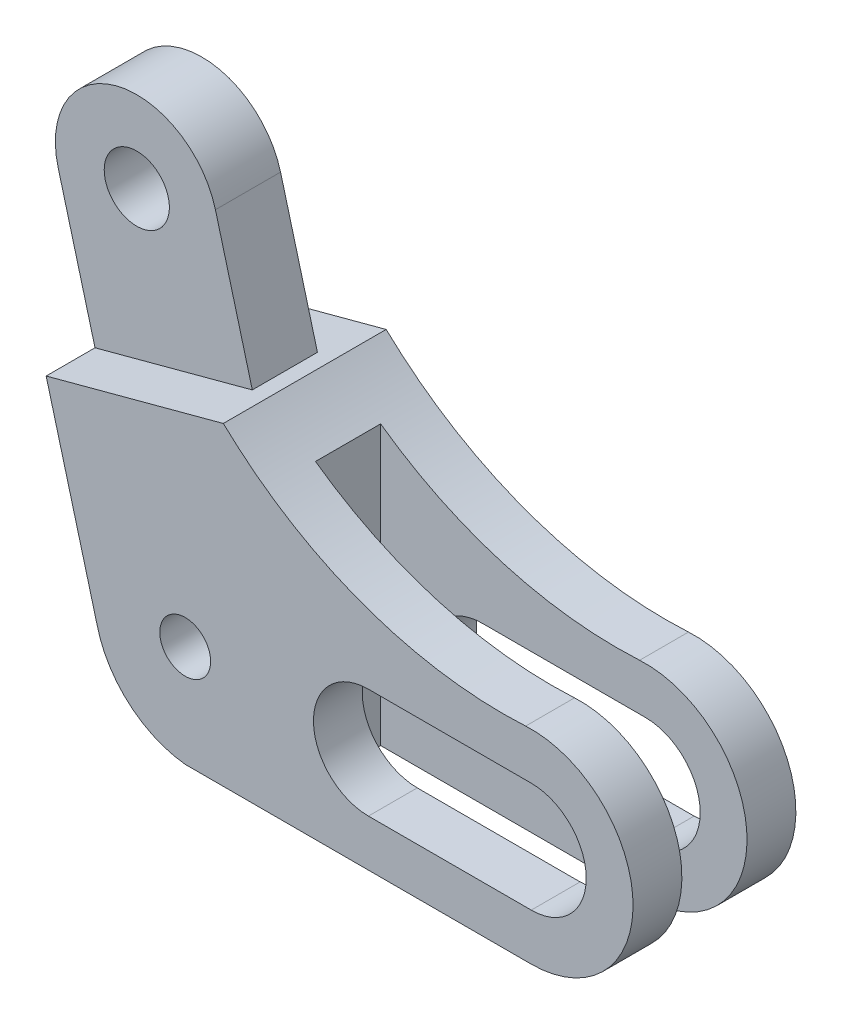
ISO-10303-21;
HEADER;
FILE_DESCRIPTION(('STEP AP214'),'2;1');
FILE_NAME('part.step','',(''),(''),'','','');
FILE_SCHEMA(('AUTOMOTIVE_DESIGN { 1 0 10303 214 1 1 1 1 }'));
ENDSEC;
DATA;
#1=APPLICATION_CONTEXT('core data for automotive mechanical design processes');
#2=APPLICATION_PROTOCOL_DEFINITION('international standard','automotive_design',2000,#1);
#3=PRODUCT_CONTEXT('',#1,'mechanical');
#4=PRODUCT('Part','Part','',(#3));
#5=PRODUCT_RELATED_PRODUCT_CATEGORY('part','',(#4));
#6=PRODUCT_DEFINITION_FORMATION('','',#4);
#7=PRODUCT_DEFINITION_CONTEXT('part definition',#1,'design');
#8=PRODUCT_DEFINITION('design','',#6,#7);
#9=PRODUCT_DEFINITION_SHAPE('','',#8);
#10=(LENGTH_UNIT() NAMED_UNIT(*) SI_UNIT(.MILLI.,.METRE.));
#11=(NAMED_UNIT(*) PLANE_ANGLE_UNIT() SI_UNIT($,.RADIAN.));
#12=(NAMED_UNIT(*) SI_UNIT($,.STERADIAN.) SOLID_ANGLE_UNIT());
#13=UNCERTAINTY_MEASURE_WITH_UNIT(LENGTH_MEASURE(1.E-05),#10,'distance_accuracy_value','');
#14=(GEOMETRIC_REPRESENTATION_CONTEXT(3) GLOBAL_UNCERTAINTY_ASSIGNED_CONTEXT((#13)) GLOBAL_UNIT_ASSIGNED_CONTEXT((#10,
#11,#12)) REPRESENTATION_CONTEXT('',''));
#15=CARTESIAN_POINT('',(0.,0.,0.));
#16=DIRECTION('',(0.,0.,1.));
#17=DIRECTION('',(1.,0.,0.));
#18=AXIS2_PLACEMENT_3D('',#15,#16,#17);
#19=CARTESIAN_POINT('',(0.,0.,20.));
#20=DIRECTION('',(0.,0.,-1.));
#21=DIRECTION('',(-1.,0.,0.));
#22=AXIS2_PLACEMENT_3D('',#19,#20,#21);
#23=CYLINDRICAL_SURFACE('',#22,25.);
#24=CARTESIAN_POINT('',(0.,0.,-8.));
#25=DIRECTION('',(0.,0.,1.));
#26=DIRECTION('',(1.,0.,0.));
#27=AXIS2_PLACEMENT_3D('',#24,#25,#26);
#28=CIRCLE('',#27,25.);
#29=CARTESIAN_POINT('',(0.,-25.,-8.));
#30=VERTEX_POINT('',#29);
#31=CARTESIAN_POINT('',(-1.37615473662768,24.9620952273814,-8.));
#32=VERTEX_POINT('',#31);
#33=EDGE_CURVE('E232',#30,#32,#28,.T.);
#34=ORIENTED_EDGE('',*,*,#33,.F.);
#35=DIRECTION('',(0.,0.,-1.));
#36=VECTOR('',#35,1.);
#37=CARTESIAN_POINT('',(0.,-25.,20.));
#38=LINE('',#37,#36);
#39=CARTESIAN_POINT('',(0.,-25.,-20.));
#40=VERTEX_POINT('',#39);
#41=EDGE_CURVE('E330',#30,#40,#38,.T.);
#42=ORIENTED_EDGE('',*,*,#41,.T.);
#43=CARTESIAN_POINT('',(0.,0.,-20.));
#44=DIRECTION('',(0.,0.,1.));
#45=DIRECTION('',(1.,0.,0.));
#46=AXIS2_PLACEMENT_3D('',#43,#44,#45);
#47=CIRCLE('',#46,25.);
#48=CARTESIAN_POINT('',(-1.37615473662768,24.9620952273814,-20.));
#49=VERTEX_POINT('',#48);
#50=EDGE_CURVE('E309',#40,#49,#47,.T.);
#51=ORIENTED_EDGE('',*,*,#50,.T.);
#52=DIRECTION('',(0.,0.,-1.));
#53=VECTOR('',#52,1.);
#54=CARTESIAN_POINT('',(-1.37615473662768,24.9620952273814,20.));
#55=LINE('',#54,#53);
#56=EDGE_CURVE('E355',#32,#49,#55,.T.);
#57=ORIENTED_EDGE('',*,*,#56,.F.);
#58=EDGE_LOOP('',(#34,#42,#51,#57));
#59=FACE_BOUND('',#58,.T.);
#60=ADVANCED_FACE('F39',(#59),#23,.T.);
#61=CARTESIAN_POINT('',(-6.88077368313851,124.810476136907,20.));
#62=DIRECTION('',(0.,0.,-1.));
#63=DIRECTION('',(-1.,0.,0.));
#64=AXIS2_PLACEMENT_3D('',#61,#62,#63);
#65=CYLINDRICAL_SURFACE('',#64,100.);
#66=CARTESIAN_POINT('',(-6.88077368313851,124.810476136907,-8.));
#67=DIRECTION('',(0.,0.,-1.));
#68=DIRECTION('',(1.,0.,0.));
#69=AXIS2_PLACEMENT_3D('',#66,#67,#68);
#70=CIRCLE('',#69,100.);
#71=CARTESIAN_POINT('',(-65.,43.433848458381,-8.));
#72=VERTEX_POINT('',#71);
#73=EDGE_CURVE('E223',#32,#72,#70,.T.);
#74=ORIENTED_EDGE('',*,*,#73,.F.);
#75=ORIENTED_EDGE('',*,*,#56,.T.);
#76=CARTESIAN_POINT('',(-6.88077368313851,124.810476136907,-20.));
#77=DIRECTION('',(0.,0.,-1.));
#78=DIRECTION('',(-1.,0.,0.));
#79=AXIS2_PLACEMENT_3D('',#76,#77,#78);
#80=CIRCLE('',#79,100.);
#81=CARTESIAN_POINT('',(-75.6404006582522,52.2011537447842,-20.));
#82=VERTEX_POINT('',#81);
#83=EDGE_CURVE('E329',#49,#82,#80,.T.);
#84=ORIENTED_EDGE('',*,*,#83,.T.);
#85=DIRECTION('',(0.,0.,-1.));
#86=VECTOR('',#85,1.);
#87=CARTESIAN_POINT('',(-75.6404006582522,52.2011537447842,20.));
#88=LINE('',#87,#86);
#89=CARTESIAN_POINT('',(-75.6404006582522,52.2011537447842,20.));
#90=VERTEX_POINT('',#89);
#91=EDGE_CURVE('E353',#90,#82,#88,.T.);
#92=ORIENTED_EDGE('',*,*,#91,.F.);
#93=CARTESIAN_POINT('',(-6.88077368313851,124.810476136907,20.));
#94=DIRECTION('',(0.,0.,-1.));
#95=DIRECTION('',(-1.,0.,0.));
#96=AXIS2_PLACEMENT_3D('',#93,#94,#95);
#97=CIRCLE('',#96,100.);
#98=CARTESIAN_POINT('',(-1.37615473662768,24.9620952273814,20.));
#99=VERTEX_POINT('',#98);
#100=EDGE_CURVE('E316',#99,#90,#97,.T.);
#101=ORIENTED_EDGE('',*,*,#100,.F.);
#102=CARTESIAN_POINT('',(-1.37615473662768,24.9620952273814,8.));
#103=VERTEX_POINT('',#102);
#104=EDGE_CURVE('E351',#99,#103,#55,.T.);
#105=ORIENTED_EDGE('',*,*,#104,.T.);
#106=CARTESIAN_POINT('',(-6.88077368313851,124.810476136907,8.));
#107=DIRECTION('',(0.,0.,-1.));
#108=DIRECTION('',(1.,0.,0.));
#109=AXIS2_PLACEMENT_3D('',#106,#107,#108);
#110=CIRCLE('',#109,100.);
#111=CARTESIAN_POINT('',(-65.,43.433848458381,8.));
#112=VERTEX_POINT('',#111);
#113=EDGE_CURVE('E193',#103,#112,#110,.T.);
#114=ORIENTED_EDGE('',*,*,#113,.T.);
#115=DIRECTION('',(0.,0.,1.));
#116=VECTOR('',#115,1.);
#117=CARTESIAN_POINT('',(-65.,43.433848458381,-8.));
#118=LINE('',#117,#116);
#119=EDGE_CURVE('E237',#72,#112,#118,.T.);
#120=ORIENTED_EDGE('',*,*,#119,.F.);
#121=EDGE_LOOP('',(#74,#75,#84,#92,#101,#105,#114,#120));
#122=FACE_BOUND('',#121,.T.);
#123=ADVANCED_FACE('F396',(#122),#65,.F.);
#124=CARTESIAN_POINT('',(0.,-25.,20.));
#125=DIRECTION('',(0.,1.,0.));
#126=DIRECTION('',(-1.,0.,0.));
#127=AXIS2_PLACEMENT_3D('',#124,#125,#126);
#128=PLANE('',#127);
#129=DIRECTION('',(1.,0.,0.));
#130=VECTOR('',#129,1.);
#131=CARTESIAN_POINT('',(-65.,-25.,-8.));
#132=LINE('',#131,#130);
#133=CARTESIAN_POINT('',(-65.,-25.,-8.));
#134=VERTEX_POINT('',#133);
#135=EDGE_CURVE('E235',#134,#30,#132,.T.);
#136=ORIENTED_EDGE('',*,*,#135,.F.);
#137=DIRECTION('',(0.,0.,1.));
#138=VECTOR('',#137,1.);
#139=CARTESIAN_POINT('',(-65.,-25.,-8.));
#140=LINE('',#139,#138);
#141=CARTESIAN_POINT('',(-65.,-25.,8.));
#142=VERTEX_POINT('',#141);
#143=EDGE_CURVE('E250',#134,#142,#140,.T.);
#144=ORIENTED_EDGE('',*,*,#143,.T.);
#145=DIRECTION('',(1.,0.,0.));
#146=VECTOR('',#145,1.);
#147=CARTESIAN_POINT('',(-65.,-25.,8.));
#148=LINE('',#147,#146);
#149=CARTESIAN_POINT('',(0.,-25.,8.));
#150=VERTEX_POINT('',#149);
#151=EDGE_CURVE('E244',#142,#150,#148,.T.);
#152=ORIENTED_EDGE('',*,*,#151,.T.);
#153=CARTESIAN_POINT('',(0.,-25.,20.));
#154=VERTEX_POINT('',#153);
#155=EDGE_CURVE('E336',#154,#150,#38,.T.);
#156=ORIENTED_EDGE('',*,*,#155,.F.);
#157=DIRECTION('',(1.,0.,0.));
#158=VECTOR('',#157,1.);
#159=CARTESIAN_POINT('',(0.,-25.,20.));
#160=LINE('',#159,#158);
#161=CARTESIAN_POINT('',(-85.,-25.,20.));
#162=VERTEX_POINT('',#161);
#163=EDGE_CURVE('E324',#162,#154,#160,.T.);
#164=ORIENTED_EDGE('',*,*,#163,.F.);
#165=DIRECTION('',(0.,0.,-1.));
#166=VECTOR('',#165,1.);
#167=CARTESIAN_POINT('',(-85.,-25.,20.));
#168=LINE('',#167,#166);
#169=CARTESIAN_POINT('',(-85.,-25.,-20.));
#170=VERTEX_POINT('',#169);
#171=EDGE_CURVE('E343',#162,#170,#168,.T.);
#172=ORIENTED_EDGE('',*,*,#171,.T.);
#173=DIRECTION('',(1.,0.,0.));
#174=VECTOR('',#173,1.);
#175=CARTESIAN_POINT('',(0.,-25.,-20.));
#176=LINE('',#175,#174);
#177=EDGE_CURVE('E320',#170,#40,#176,.T.);
#178=ORIENTED_EDGE('',*,*,#177,.T.);
#179=ORIENTED_EDGE('',*,*,#41,.F.);
#180=EDGE_LOOP('',(#136,#144,#152,#156,#164,#172,#178,#179));
#181=FACE_BOUND('',#180,.T.);
#182=ADVANCED_FACE('F405',(#181),#128,.F.);
#183=CARTESIAN_POINT('',(-40.,0.,-20.));
#184=DIRECTION('',(0.,0.,1.));
#185=DIRECTION('',(1.,0.,0.));
#186=AXIS2_PLACEMENT_3D('',#183,#184,#185);
#187=CYLINDRICAL_SURFACE('',#186,13.5);
#188=CARTESIAN_POINT('',(-40.,0.,-8.));
#189=DIRECTION('',(0.,0.,1.));
#190=DIRECTION('',(1.,0.,0.));
#191=AXIS2_PLACEMENT_3D('',#188,#189,#190);
#192=CIRCLE('',#191,13.5);
#193=CARTESIAN_POINT('',(-40.,-13.5,-8.));
#194=VERTEX_POINT('',#193);
#195=CARTESIAN_POINT('',(-40.,13.5,-8.));
#196=VERTEX_POINT('',#195);
#197=EDGE_CURVE('E262',#194,#196,#192,.F.);
#198=ORIENTED_EDGE('',*,*,#197,.F.);
#199=DIRECTION('',(0.,0.,1.));
#200=VECTOR('',#199,1.);
#201=CARTESIAN_POINT('',(-40.,-13.5,-20.));
#202=LINE('',#201,#200);
#203=CARTESIAN_POINT('',(-40.,-13.5,-20.));
#204=VERTEX_POINT('',#203);
#205=EDGE_CURVE('E302',#204,#194,#202,.T.);
#206=ORIENTED_EDGE('',*,*,#205,.F.);
#207=CARTESIAN_POINT('',(-40.,0.,-20.));
#208=DIRECTION('',(0.,0.,1.));
#209=DIRECTION('',(1.,0.,0.));
#210=AXIS2_PLACEMENT_3D('',#207,#208,#209);
#211=CIRCLE('',#210,13.5);
#212=CARTESIAN_POINT('',(-40.,13.5,-20.));
#213=VERTEX_POINT('',#212);
#214=EDGE_CURVE('E270',#213,#204,#211,.T.);
#215=ORIENTED_EDGE('',*,*,#214,.F.);
#216=DIRECTION('',(0.,0.,1.));
#217=VECTOR('',#216,1.);
#218=CARTESIAN_POINT('',(-40.,13.5,-20.));
#219=LINE('',#218,#217);
#220=EDGE_CURVE('E292',#213,#196,#219,.T.);
#221=ORIENTED_EDGE('',*,*,#220,.T.);
#222=EDGE_LOOP('',(#198,#206,#215,#221));
#223=FACE_BOUND('',#222,.T.);
#224=ADVANCED_FACE('F393',(#223),#187,.F.);
#225=CARTESIAN_POINT('',(-40.,13.5,-20.));
#226=DIRECTION('',(0.,1.,0.));
#227=DIRECTION('',(0.,0.,1.));
#228=AXIS2_PLACEMENT_3D('',#225,#226,#227);
#229=PLANE('',#228);
#230=DIRECTION('',(1.,0.,0.));
#231=VECTOR('',#230,1.);
#232=CARTESIAN_POINT('',(-40.,13.5,-8.));
#233=LINE('',#232,#231);
#234=CARTESIAN_POINT('',(0.,13.5,-8.));
#235=VERTEX_POINT('',#234);
#236=EDGE_CURVE('E265',#196,#235,#233,.T.);
#237=ORIENTED_EDGE('',*,*,#236,.F.);
#238=ORIENTED_EDGE('',*,*,#220,.F.);
#239=DIRECTION('',(-1.,0.,0.));
#240=VECTOR('',#239,1.);
#241=CARTESIAN_POINT('',(-40.,13.5,-20.));
#242=LINE('',#241,#240);
#243=CARTESIAN_POINT('',(0.,13.5,-20.));
#244=VERTEX_POINT('',#243);
#245=EDGE_CURVE('E280',#244,#213,#242,.T.);
#246=ORIENTED_EDGE('',*,*,#245,.F.);
#247=DIRECTION('',(0.,0.,1.));
#248=VECTOR('',#247,1.);
#249=CARTESIAN_POINT('',(0.,13.5,-20.));
#250=LINE('',#249,#248);
#251=EDGE_CURVE('E298',#244,#235,#250,.T.);
#252=ORIENTED_EDGE('',*,*,#251,.T.);
#253=EDGE_LOOP('',(#237,#238,#246,#252));
#254=FACE_BOUND('',#253,.T.);
#255=ADVANCED_FACE('F385',(#254),#229,.F.);
#256=CARTESIAN_POINT('',(0.,0.,-20.));
#257=DIRECTION('',(0.,0.,1.));
#258=DIRECTION('',(1.,0.,0.));
#259=AXIS2_PLACEMENT_3D('',#256,#257,#258);
#260=CYLINDRICAL_SURFACE('',#259,13.5);
#261=CARTESIAN_POINT('',(0.,0.,-8.));
#262=DIRECTION('',(0.,0.,1.));
#263=DIRECTION('',(1.,0.,0.));
#264=AXIS2_PLACEMENT_3D('',#261,#262,#263);
#265=CIRCLE('',#264,13.5);
#266=CARTESIAN_POINT('',(0.,-13.5,-8.));
#267=VERTEX_POINT('',#266);
#268=EDGE_CURVE('E257',#235,#267,#265,.F.);
#269=ORIENTED_EDGE('',*,*,#268,.F.);
#270=ORIENTED_EDGE('',*,*,#251,.F.);
#271=CARTESIAN_POINT('',(0.,0.,-20.));
#272=DIRECTION('',(0.,0.,1.));
#273=DIRECTION('',(1.,0.,0.));
#274=AXIS2_PLACEMENT_3D('',#271,#272,#273);
#275=CIRCLE('',#274,13.5);
#276=CARTESIAN_POINT('',(0.,-13.5,-20.));
#277=VERTEX_POINT('',#276);
#278=EDGE_CURVE('E273',#277,#244,#275,.T.);
#279=ORIENTED_EDGE('',*,*,#278,.F.);
#280=DIRECTION('',(0.,0.,1.));
#281=VECTOR('',#280,1.);
#282=CARTESIAN_POINT('',(0.,-13.5,-20.));
#283=LINE('',#282,#281);
#284=EDGE_CURVE('E296',#277,#267,#283,.T.);
#285=ORIENTED_EDGE('',*,*,#284,.T.);
#286=EDGE_LOOP('',(#269,#270,#279,#285));
#287=FACE_BOUND('',#286,.T.);
#288=ADVANCED_FACE('F389',(#287),#260,.F.);
#289=CARTESIAN_POINT('',(-40.,-13.5,-20.));
#290=DIRECTION('',(0.,-1.,0.));
#291=DIRECTION('',(0.,0.,-1.));
#292=AXIS2_PLACEMENT_3D('',#289,#290,#291);
#293=PLANE('',#292);
#294=DIRECTION('',(-1.,0.,0.));
#295=VECTOR('',#294,1.);
#296=CARTESIAN_POINT('',(-40.,-13.5,-8.));
#297=LINE('',#296,#295);
#298=EDGE_CURVE('E11',#267,#194,#297,.T.);
#299=ORIENTED_EDGE('',*,*,#298,.F.);
#300=ORIENTED_EDGE('',*,*,#284,.F.);
#301=DIRECTION('',(1.,0.,0.));
#302=VECTOR('',#301,1.);
#303=CARTESIAN_POINT('',(-40.,-13.5,-20.));
#304=LINE('',#303,#302);
#305=EDGE_CURVE('E269',#204,#277,#304,.T.);
#306=ORIENTED_EDGE('',*,*,#305,.F.);
#307=ORIENTED_EDGE('',*,*,#205,.T.);
#308=EDGE_LOOP('',(#299,#300,#306,#307));
#309=FACE_BOUND('',#308,.T.);
#310=ADVANCED_FACE('F462',(#309),#293,.F.);
#311=CARTESIAN_POINT('',(0.,0.,20.));
#312=DIRECTION('',(0.,0.,1.));
#313=DIRECTION('',(1.,0.,0.));
#314=AXIS2_PLACEMENT_3D('',#311,#312,#313);
#315=PLANE('',#314);
#316=CARTESIAN_POINT('',(-40.,0.,20.));
#317=DIRECTION('',(0.,0.,1.));
#318=DIRECTION('',(1.,0.,0.));
#319=AXIS2_PLACEMENT_3D('',#316,#317,#318);
#320=CIRCLE('',#319,13.5);
#321=CARTESIAN_POINT('',(-40.,13.5,20.));
#322=VERTEX_POINT('',#321);
#323=CARTESIAN_POINT('',(-40.,-13.5,20.));
#324=VERTEX_POINT('',#323);
#325=EDGE_CURVE('E266',#322,#324,#320,.T.);
#326=ORIENTED_EDGE('',*,*,#325,.F.);
#327=DIRECTION('',(-1.,0.,0.));
#328=VECTOR('',#327,1.);
#329=CARTESIAN_POINT('',(-40.,13.5,20.));
#330=LINE('',#329,#328);
#331=CARTESIAN_POINT('',(0.,13.5,20.));
#332=VERTEX_POINT('',#331);
#333=EDGE_CURVE('E271',#332,#322,#330,.T.);
#334=ORIENTED_EDGE('',*,*,#333,.F.);
#335=CARTESIAN_POINT('',(0.,0.,20.));
#336=DIRECTION('',(0.,0.,1.));
#337=DIRECTION('',(1.,0.,0.));
#338=AXIS2_PLACEMENT_3D('',#335,#336,#337);
#339=CIRCLE('',#338,13.5);
#340=CARTESIAN_POINT('',(0.,-13.5,20.));
#341=VERTEX_POINT('',#340);
#342=EDGE_CURVE('E286',#341,#332,#339,.T.);
#343=ORIENTED_EDGE('',*,*,#342,.F.);
#344=DIRECTION('',(1.,0.,0.));
#345=VECTOR('',#344,1.);
#346=CARTESIAN_POINT('',(-40.,-13.5,20.));
#347=LINE('',#346,#345);
#348=EDGE_CURVE('E282',#324,#341,#347,.T.);
#349=ORIENTED_EDGE('',*,*,#348,.F.);
#350=EDGE_LOOP('',(#326,#334,#343,#349));
#351=FACE_BOUND('',#350,.T.);
#352=CARTESIAN_POINT('',(0.,0.,20.));
#353=DIRECTION('',(0.,0.,1.));
#354=DIRECTION('',(1.,0.,0.));
#355=AXIS2_PLACEMENT_3D('',#352,#353,#354);
#356=CIRCLE('',#355,25.);
#357=EDGE_CURVE('E311',#154,#99,#356,.T.);
#358=ORIENTED_EDGE('',*,*,#357,.T.);
#359=ORIENTED_EDGE('',*,*,#100,.T.);
#360=DIRECTION('',(-0.965925826289068,-0.258819045102521,0.));
#361=VECTOR('',#360,1.);
#362=CARTESIAN_POINT('',(-119.156645256425,40.5410111470685,20.));
#363=LINE('',#362,#361);
#364=CARTESIAN_POINT('',(-119.156645256425,40.5410111470685,20.));
#365=VERTEX_POINT('',#364);
#366=EDGE_CURVE('E317',#90,#365,#363,.T.);
#367=ORIENTED_EDGE('',*,*,#366,.T.);
#368=DIRECTION('',(0.258819045102522,-0.965925826289068,0.));
#369=VECTOR('',#368,1.);
#370=CARTESIAN_POINT('',(-106.733331091504,-5.82342851480675,20.));
#371=LINE('',#370,#369);
#372=CARTESIAN_POINT('',(-106.733331091504,-5.82342851480675,20.));
#373=VERTEX_POINT('',#372);
#374=EDGE_CURVE('E321',#365,#373,#371,.T.);
#375=ORIENTED_EDGE('',*,*,#374,.T.);
#376=CARTESIAN_POINT('',(-82.3886864264471,-0.136753200344534,20.));
#377=DIRECTION('',(0.,0.,1.));
#378=DIRECTION('',(-1.,0.,0.));
#379=AXIS2_PLACEMENT_3D('',#376,#377,#378);
#380=CIRCLE('',#379,25.);
#381=EDGE_CURVE('E323',#373,#162,#380,.T.);
#382=ORIENTED_EDGE('',*,*,#381,.T.);
#383=ORIENTED_EDGE('',*,*,#163,.T.);
#384=EDGE_LOOP('',(#358,#359,#367,#375,#382,#383));
#385=FACE_BOUND('',#384,.T.);
#386=CARTESIAN_POINT('',(-85.,0.,20.));
#387=DIRECTION('',(0.,0.,1.));
#388=DIRECTION('',(1.,0.,0.));
#389=AXIS2_PLACEMENT_3D('',#386,#387,#388);
#390=CIRCLE('',#389,6.25);
#391=CARTESIAN_POINT('',(-78.75,0.,20.));
#392=VERTEX_POINT('',#391);
#393=EDGE_CURVE('E307',#392,#392,#390,.T.);
#394=ORIENTED_EDGE('',*,*,#393,.F.);
#395=EDGE_LOOP('',(#394));
#396=FACE_BOUND('',#395,.T.);
#397=ADVANCED_FACE('F375',(#351,#385,#396),#315,.T.);
#398=CARTESIAN_POINT('',(0.,0.,-20.));
#399=DIRECTION('',(0.,0.,1.));
#400=DIRECTION('',(1.,0.,0.));
#401=AXIS2_PLACEMENT_3D('',#398,#399,#400);
#402=PLANE('',#401);
#403=ORIENTED_EDGE('',*,*,#245,.T.);
#404=ORIENTED_EDGE('',*,*,#214,.T.);
#405=ORIENTED_EDGE('',*,*,#305,.T.);
#406=ORIENTED_EDGE('',*,*,#278,.T.);
#407=EDGE_LOOP('',(#403,#404,#405,#406));
#408=FACE_BOUND('',#407,.T.);
#409=ORIENTED_EDGE('',*,*,#50,.F.);
#410=ORIENTED_EDGE('',*,*,#177,.F.);
#411=CARTESIAN_POINT('',(-82.3886864264471,-0.136753200344534,-20.));
#412=DIRECTION('',(0.,0.,1.));
#413=DIRECTION('',(-1.,0.,0.));
#414=AXIS2_PLACEMENT_3D('',#411,#412,#413);
#415=CIRCLE('',#414,25.);
#416=CARTESIAN_POINT('',(-106.733331091504,-5.82342851480675,-20.));
#417=VERTEX_POINT('',#416);
#418=EDGE_CURVE('E338',#417,#170,#415,.T.);
#419=ORIENTED_EDGE('',*,*,#418,.F.);
#420=DIRECTION('',(0.258819045102522,-0.965925826289068,0.));
#421=VECTOR('',#420,1.);
#422=CARTESIAN_POINT('',(-106.733331091504,-5.82342851480675,-20.));
#423=LINE('',#422,#421);
#424=CARTESIAN_POINT('',(-119.156645256425,40.5410111470685,-20.));
#425=VERTEX_POINT('',#424);
#426=EDGE_CURVE('E331',#425,#417,#423,.T.);
#427=ORIENTED_EDGE('',*,*,#426,.F.);
#428=DIRECTION('',(-0.965925826289068,-0.258819045102521,0.));
#429=VECTOR('',#428,1.);
#430=CARTESIAN_POINT('',(-119.156645256425,40.5410111470685,-20.));
#431=LINE('',#430,#429);
#432=EDGE_CURVE('E335',#82,#425,#431,.T.);
#433=ORIENTED_EDGE('',*,*,#432,.F.);
#434=ORIENTED_EDGE('',*,*,#83,.F.);
#435=EDGE_LOOP('',(#409,#410,#419,#427,#433,#434));
#436=FACE_BOUND('',#435,.T.);
#437=CARTESIAN_POINT('',(-85.,0.,-20.));
#438=DIRECTION('',(0.,0.,1.));
#439=DIRECTION('',(1.,0.,0.));
#440=AXIS2_PLACEMENT_3D('',#437,#438,#439);
#441=CIRCLE('',#440,6.25);
#442=CARTESIAN_POINT('',(-78.75,0.,-20.));
#443=VERTEX_POINT('',#442);
#444=EDGE_CURVE('E294',#443,#443,#441,.T.);
#445=ORIENTED_EDGE('',*,*,#444,.T.);
#446=EDGE_LOOP('',(#445));
#447=FACE_BOUND('',#446,.T.);
#448=ADVANCED_FACE('F408',(#408,#436,#447),#402,.F.);
#449=ORIENTED_EDGE('',*,*,#155,.T.);
#450=CARTESIAN_POINT('',(0.,0.,8.));
#451=DIRECTION('',(0.,0.,1.));
#452=DIRECTION('',(1.,0.,0.));
#453=AXIS2_PLACEMENT_3D('',#450,#451,#452);
#454=CIRCLE('',#453,25.);
#455=EDGE_CURVE('E230',#150,#103,#454,.T.);
#456=ORIENTED_EDGE('',*,*,#455,.T.);
#457=ORIENTED_EDGE('',*,*,#104,.F.);
#458=ORIENTED_EDGE('',*,*,#357,.F.);
#459=EDGE_LOOP('',(#449,#456,#457,#458));
#460=FACE_BOUND('',#459,.T.);
#461=ADVANCED_FACE('F41',(#460),#23,.T.);
#462=CARTESIAN_POINT('',(-119.156645256425,40.5410111470685,20.));
#463=DIRECTION('',(0.258819045102521,-0.965925826289068,0.));
#464=DIRECTION('',(0.965925826289068,0.258819045102521,0.));
#465=AXIS2_PLACEMENT_3D('',#462,#463,#464);
#466=PLANE('',#465);
#467=DIRECTION('',(0.,0.,-1.));
#468=VECTOR('',#467,1.);
#469=CARTESIAN_POINT('',(-119.156645256425,40.5410111470685,20.));
#470=LINE('',#469,#468);
#471=CARTESIAN_POINT('',(-119.156645256425,40.5410111470685,-8.));
#472=VERTEX_POINT('',#471);
#473=EDGE_CURVE('E58',#472,#425,#470,.T.);
#474=ORIENTED_EDGE('',*,*,#473,.F.);
#475=DIRECTION('',(0.965925826289068,0.258819045102521,0.));
#476=VECTOR('',#475,1.);
#477=CARTESIAN_POINT('',(-80.5196122048624,50.8937729511694,-8.));
#478=LINE('',#477,#476);
#479=CARTESIAN_POINT('',(-80.5196122048624,50.8937729511694,-8.));
#480=VERTEX_POINT('',#479);
#481=EDGE_CURVE('E54',#472,#480,#478,.T.);
#482=ORIENTED_EDGE('',*,*,#481,.T.);
#483=DIRECTION('',(0.,0.,-1.));
#484=VECTOR('',#483,1.);
#485=CARTESIAN_POINT('',(-80.5196122048624,50.8937729511694,8.));
#486=LINE('',#485,#484);
#487=CARTESIAN_POINT('',(-80.5196122048624,50.8937729511694,8.));
#488=VERTEX_POINT('',#487);
#489=EDGE_CURVE('E183',#488,#480,#486,.T.);
#490=ORIENTED_EDGE('',*,*,#489,.F.);
#491=DIRECTION('',(0.965925826289068,0.258819045102521,0.));
#492=VECTOR('',#491,1.);
#493=CARTESIAN_POINT('',(-80.5196122048624,50.8937729511694,8.));
#494=LINE('',#493,#492);
#495=CARTESIAN_POINT('',(-119.156645256425,40.5410111470685,8.));
#496=VERTEX_POINT('',#495);
#497=EDGE_CURVE('E186',#496,#488,#494,.T.);
#498=ORIENTED_EDGE('',*,*,#497,.F.);
#499=EDGE_CURVE('E349',#365,#496,#470,.T.);
#500=ORIENTED_EDGE('',*,*,#499,.F.);
#501=ORIENTED_EDGE('',*,*,#366,.F.);
#502=ORIENTED_EDGE('',*,*,#91,.T.);
#503=ORIENTED_EDGE('',*,*,#432,.T.);
#504=EDGE_LOOP('',(#474,#482,#490,#498,#500,#501,#502,#503));
#505=FACE_BOUND('',#504,.T.);
#506=ADVANCED_FACE('F189',(#505),#466,.F.);
#507=CARTESIAN_POINT('',(-106.733331091504,-5.82342851480675,20.));
#508=DIRECTION('',(0.965925826289068,0.258819045102522,0.));
#509=DIRECTION('',(-0.258819045102522,0.965925826289068,0.));
#510=AXIS2_PLACEMENT_3D('',#507,#508,#509);
#511=PLANE('',#510);
#512=ORIENTED_EDGE('',*,*,#426,.T.);
#513=DIRECTION('',(0.,0.,-1.));
#514=VECTOR('',#513,1.);
#515=CARTESIAN_POINT('',(-106.733331091504,-5.82342851480675,20.));
#516=LINE('',#515,#514);
#517=EDGE_CURVE('E347',#373,#417,#516,.T.);
#518=ORIENTED_EDGE('',*,*,#517,.F.);
#519=ORIENTED_EDGE('',*,*,#374,.F.);
#520=ORIENTED_EDGE('',*,*,#499,.T.);
#521=DIRECTION('',(0.258819045102522,-0.965925826289068,0.));
#522=VECTOR('',#521,1.);
#523=CARTESIAN_POINT('',(-119.156645256425,40.5410111470685,8.));
#524=LINE('',#523,#522);
#525=CARTESIAN_POINT('',(-128.215311835013,74.348415067186,8.));
#526=VERTEX_POINT('',#525);
#527=EDGE_CURVE('E210',#526,#496,#524,.T.);
#528=ORIENTED_EDGE('',*,*,#527,.F.);
#529=DIRECTION('',(0.,0.,-1.));
#530=VECTOR('',#529,1.);
#531=CARTESIAN_POINT('',(-128.215311835013,74.348415067186,8.));
#532=LINE('',#531,#530);
#533=CARTESIAN_POINT('',(-128.215311835013,74.348415067186,-8.));
#534=VERTEX_POINT('',#533);
#535=EDGE_CURVE('E220',#526,#534,#532,.T.);
#536=ORIENTED_EDGE('',*,*,#535,.T.);
#537=DIRECTION('',(0.258819045102522,-0.965925826289068,0.));
#538=VECTOR('',#537,1.);
#539=CARTESIAN_POINT('',(-119.156645256425,40.5410111470685,-8.));
#540=LINE('',#539,#538);
#541=EDGE_CURVE('E208',#534,#472,#540,.T.);
#542=ORIENTED_EDGE('',*,*,#541,.T.);
#543=ORIENTED_EDGE('',*,*,#473,.T.);
#544=EDGE_LOOP('',(#512,#518,#519,#520,#528,#536,#542,#543));
#545=FACE_BOUND('',#544,.T.);
#546=ADVANCED_FACE('F415',(#545),#511,.F.);
#547=CARTESIAN_POINT('',(-82.3886864264471,-0.136753200344534,20.));
#548=DIRECTION('',(0.,0.,-1.));
#549=DIRECTION('',(-1.,0.,0.));
#550=AXIS2_PLACEMENT_3D('',#547,#548,#549);
#551=CYLINDRICAL_SURFACE('',#550,25.);
#552=ORIENTED_EDGE('',*,*,#418,.T.);
#553=ORIENTED_EDGE('',*,*,#171,.F.);
#554=ORIENTED_EDGE('',*,*,#381,.F.);
#555=ORIENTED_EDGE('',*,*,#517,.T.);
#556=EDGE_LOOP('',(#552,#553,#554,#555));
#557=FACE_BOUND('',#556,.T.);
#558=ADVANCED_FACE('F440',(#557),#551,.T.);
#559=CARTESIAN_POINT('',(-85.,0.,20.));
#560=DIRECTION('',(0.,0.,-1.));
#561=DIRECTION('',(-1.,0.,0.));
#562=AXIS2_PLACEMENT_3D('',#559,#560,#561);
#563=CYLINDRICAL_SURFACE('',#562,6.25);
#564=ORIENTED_EDGE('',*,*,#393,.T.);
#565=EDGE_LOOP('',(#564));
#566=FACE_BOUND('',#565,.T.);
#567=ORIENTED_EDGE('',*,*,#444,.F.);
#568=EDGE_LOOP('',(#567));
#569=FACE_BOUND('',#568,.T.);
#570=ADVANCED_FACE('F386',(#566,#569),#563,.F.);
#571=CARTESIAN_POINT('',(-40.,-13.5,8.));
#572=VERTEX_POINT('',#571);
#573=EDGE_CURVE('E278',#572,#324,#202,.T.);
#574=ORIENTED_EDGE('',*,*,#573,.F.);
#575=CARTESIAN_POINT('',(-40.,0.,8.));
#576=DIRECTION('',(0.,0.,1.));
#577=DIRECTION('',(1.,0.,0.));
#578=AXIS2_PLACEMENT_3D('',#575,#576,#577);
#579=CIRCLE('',#578,13.5);
#580=CARTESIAN_POINT('',(-40.,13.5,8.));
#581=VERTEX_POINT('',#580);
#582=EDGE_CURVE('E260',#572,#581,#579,.F.);
#583=ORIENTED_EDGE('',*,*,#582,.T.);
#584=EDGE_CURVE('E293',#581,#322,#219,.T.);
#585=ORIENTED_EDGE('',*,*,#584,.T.);
#586=ORIENTED_EDGE('',*,*,#325,.T.);
#587=EDGE_LOOP('',(#574,#583,#585,#586));
#588=FACE_BOUND('',#587,.T.);
#589=ADVANCED_FACE('F364',(#588),#187,.F.);
#590=ORIENTED_EDGE('',*,*,#584,.F.);
#591=DIRECTION('',(1.,0.,0.));
#592=VECTOR('',#591,1.);
#593=CARTESIAN_POINT('',(-40.,13.5,8.));
#594=LINE('',#593,#592);
#595=CARTESIAN_POINT('',(0.,13.5,8.));
#596=VERTEX_POINT('',#595);
#597=EDGE_CURVE('E255',#581,#596,#594,.T.);
#598=ORIENTED_EDGE('',*,*,#597,.T.);
#599=EDGE_CURVE('E300',#596,#332,#250,.T.);
#600=ORIENTED_EDGE('',*,*,#599,.T.);
#601=ORIENTED_EDGE('',*,*,#333,.T.);
#602=EDGE_LOOP('',(#590,#598,#600,#601));
#603=FACE_BOUND('',#602,.T.);
#604=ADVANCED_FACE('F377',(#603),#229,.F.);
#605=ORIENTED_EDGE('',*,*,#599,.F.);
#606=CARTESIAN_POINT('',(0.,0.,8.));
#607=DIRECTION('',(0.,0.,1.));
#608=DIRECTION('',(1.,0.,0.));
#609=AXIS2_PLACEMENT_3D('',#606,#607,#608);
#610=CIRCLE('',#609,13.5);
#611=CARTESIAN_POINT('',(0.,-13.5,8.));
#612=VERTEX_POINT('',#611);
#613=EDGE_CURVE('E249',#596,#612,#610,.F.);
#614=ORIENTED_EDGE('',*,*,#613,.T.);
#615=EDGE_CURVE('E303',#612,#341,#283,.T.);
#616=ORIENTED_EDGE('',*,*,#615,.T.);
#617=ORIENTED_EDGE('',*,*,#342,.T.);
#618=EDGE_LOOP('',(#605,#614,#616,#617));
#619=FACE_BOUND('',#618,.T.);
#620=ADVANCED_FACE('F376',(#619),#260,.F.);
#621=ORIENTED_EDGE('',*,*,#615,.F.);
#622=DIRECTION('',(-1.,0.,0.));
#623=VECTOR('',#622,1.);
#624=CARTESIAN_POINT('',(-40.,-13.5,8.));
#625=LINE('',#624,#623);
#626=EDGE_CURVE('E48',#612,#572,#625,.T.);
#627=ORIENTED_EDGE('',*,*,#626,.T.);
#628=ORIENTED_EDGE('',*,*,#573,.T.);
#629=ORIENTED_EDGE('',*,*,#348,.T.);
#630=EDGE_LOOP('',(#621,#627,#628,#629));
#631=FACE_BOUND('',#630,.T.);
#632=ADVANCED_FACE('F362',(#631),#293,.F.);
#633=CARTESIAN_POINT('',(-6.88077368313851,124.810476136907,-8.));
#634=DIRECTION('',(0.,0.,1.));
#635=DIRECTION('',(1.,0.,0.));
#636=AXIS2_PLACEMENT_3D('',#633,#634,#635);
#637=PLANE('',#636);
#638=ORIENTED_EDGE('',*,*,#73,.T.);
#639=DIRECTION('',(0.,-1.,0.));
#640=VECTOR('',#639,1.);
#641=CARTESIAN_POINT('',(-65.,43.433848458381,-8.));
#642=LINE('',#641,#640);
#643=EDGE_CURVE('E227',#72,#134,#642,.T.);
#644=ORIENTED_EDGE('',*,*,#643,.T.);
#645=ORIENTED_EDGE('',*,*,#135,.T.);
#646=ORIENTED_EDGE('',*,*,#33,.T.);
#647=EDGE_LOOP('',(#638,#644,#645,#646));
#648=FACE_BOUND('',#647,.T.);
#649=ORIENTED_EDGE('',*,*,#197,.T.);
#650=ORIENTED_EDGE('',*,*,#236,.T.);
#651=ORIENTED_EDGE('',*,*,#268,.T.);
#652=ORIENTED_EDGE('',*,*,#298,.T.);
#653=EDGE_LOOP('',(#649,#650,#651,#652));
#654=FACE_BOUND('',#653,.T.);
#655=ADVANCED_FACE('F447',(#648,#654),#637,.T.);
#656=CARTESIAN_POINT('',(-6.88077368313851,124.810476136907,8.));
#657=DIRECTION('',(0.,0.,1.));
#658=DIRECTION('',(1.,0.,0.));
#659=AXIS2_PLACEMENT_3D('',#656,#657,#658);
#660=PLANE('',#659);
#661=ORIENTED_EDGE('',*,*,#113,.F.);
#662=ORIENTED_EDGE('',*,*,#455,.F.);
#663=ORIENTED_EDGE('',*,*,#151,.F.);
#664=DIRECTION('',(0.,-1.,0.));
#665=VECTOR('',#664,1.);
#666=CARTESIAN_POINT('',(-65.,43.433848458381,8.));
#667=LINE('',#666,#665);
#668=EDGE_CURVE('E239',#112,#142,#667,.T.);
#669=ORIENTED_EDGE('',*,*,#668,.F.);
#670=EDGE_LOOP('',(#661,#662,#663,#669));
#671=FACE_BOUND('',#670,.T.);
#672=ORIENTED_EDGE('',*,*,#626,.F.);
#673=ORIENTED_EDGE('',*,*,#613,.F.);
#674=ORIENTED_EDGE('',*,*,#597,.F.);
#675=ORIENTED_EDGE('',*,*,#582,.F.);
#676=EDGE_LOOP('',(#672,#673,#674,#675));
#677=FACE_BOUND('',#676,.T.);
#678=ADVANCED_FACE('F380',(#671,#677),#660,.F.);
#679=CARTESIAN_POINT('',(-65.,43.433848458381,-8.));
#680=DIRECTION('',(-1.,0.,0.));
#681=DIRECTION('',(0.,-1.,0.));
#682=AXIS2_PLACEMENT_3D('',#679,#680,#681);
#683=PLANE('',#682);
#684=ORIENTED_EDGE('',*,*,#668,.T.);
#685=ORIENTED_EDGE('',*,*,#143,.F.);
#686=ORIENTED_EDGE('',*,*,#643,.F.);
#687=ORIENTED_EDGE('',*,*,#119,.T.);
#688=EDGE_LOOP('',(#684,#685,#686,#687));
#689=FACE_BOUND('',#688,.T.);
#690=ADVANCED_FACE('F422',(#689),#683,.F.);
#691=CARTESIAN_POINT('',(-89.5782787834506,84.7011768712868,8.));
#692=DIRECTION('',(-0.965925826289068,-0.258819045102522,0.));
#693=DIRECTION('',(0.258819045102522,-0.965925826289068,0.));
#694=AXIS2_PLACEMENT_3D('',#691,#692,#693);
#695=PLANE('',#694);
#696=DIRECTION('',(-0.258819045102521,0.965925826289068,0.));
#697=VECTOR('',#696,1.);
#698=CARTESIAN_POINT('',(-89.5782787834506,84.7011768712868,-8.));
#699=LINE('',#698,#697);
#700=CARTESIAN_POINT('',(-89.5782787834506,84.7011768712868,-8.));
#701=VERTEX_POINT('',#700);
#702=EDGE_CURVE('E218',#480,#701,#699,.T.);
#703=ORIENTED_EDGE('',*,*,#702,.T.);
#704=DIRECTION('',(0.,0.,-1.));
#705=VECTOR('',#704,1.);
#706=CARTESIAN_POINT('',(-89.5782787834506,84.7011768712868,8.));
#707=LINE('',#706,#705);
#708=CARTESIAN_POINT('',(-89.5782787834506,84.7011768712868,8.));
#709=VERTEX_POINT('',#708);
#710=EDGE_CURVE('E192',#709,#701,#707,.T.);
#711=ORIENTED_EDGE('',*,*,#710,.F.);
#712=DIRECTION('',(-0.258819045102521,0.965925826289068,0.));
#713=VECTOR('',#712,1.);
#714=CARTESIAN_POINT('',(-89.5782787834506,84.7011768712868,8.));
#715=LINE('',#714,#713);
#716=EDGE_CURVE('E197',#488,#709,#715,.T.);
#717=ORIENTED_EDGE('',*,*,#716,.F.);
#718=ORIENTED_EDGE('',*,*,#489,.T.);
#719=EDGE_LOOP('',(#703,#711,#717,#718));
#720=FACE_BOUND('',#719,.T.);
#721=ADVANCED_FACE('F196',(#720),#695,.F.);
#722=CARTESIAN_POINT('',(-108.896795309232,79.5247959692363,8.));
#723=DIRECTION('',(0.,0.,-1.));
#724=DIRECTION('',(-1.,0.,0.));
#725=AXIS2_PLACEMENT_3D('',#722,#723,#724);
#726=CYLINDRICAL_SURFACE('',#725,20.);
#727=CARTESIAN_POINT('',(-108.896795309232,79.5247959692363,-8.));
#728=DIRECTION('',(0.,0.,1.));
#729=DIRECTION('',(-1.,0.,0.));
#730=AXIS2_PLACEMENT_3D('',#727,#728,#729);
#731=CIRCLE('',#730,20.);
#732=EDGE_CURVE('E209',#701,#534,#731,.T.);
#733=ORIENTED_EDGE('',*,*,#732,.T.);
#734=ORIENTED_EDGE('',*,*,#535,.F.);
#735=CARTESIAN_POINT('',(-108.896795309232,79.5247959692363,8.));
#736=DIRECTION('',(0.,0.,1.));
#737=DIRECTION('',(-1.,0.,0.));
#738=AXIS2_PLACEMENT_3D('',#735,#736,#737);
#739=CIRCLE('',#738,20.);
#740=EDGE_CURVE('E205',#709,#526,#739,.T.);
#741=ORIENTED_EDGE('',*,*,#740,.F.);
#742=ORIENTED_EDGE('',*,*,#710,.T.);
#743=EDGE_LOOP('',(#733,#734,#741,#742));
#744=FACE_BOUND('',#743,.T.);
#745=ADVANCED_FACE('F511',(#744),#726,.T.);
#746=CARTESIAN_POINT('',(-108.896795309232,79.5247959692363,8.));
#747=DIRECTION('',(0.,0.,-1.));
#748=DIRECTION('',(-1.,0.,0.));
#749=AXIS2_PLACEMENT_3D('',#746,#747,#748);
#750=PLANE('',#749);
#751=CARTESIAN_POINT('',(-108.896795309232,79.5247959692363,8.00000000000001));
#752=DIRECTION('',(0.,0.,-1.));
#753=DIRECTION('',(-1.,0.,0.));
#754=AXIS2_PLACEMENT_3D('',#751,#752,#753);
#755=CIRCLE('',#754,8.);
#756=CARTESIAN_POINT('',(-116.896795309232,79.5247959692363,8.00000000000001));
#757=VERTEX_POINT('',#756);
#758=EDGE_CURVE('E213',#757,#757,#755,.T.);
#759=ORIENTED_EDGE('',*,*,#758,.T.);
#760=EDGE_LOOP('',(#759));
#761=FACE_BOUND('',#760,.T.);
#762=ORIENTED_EDGE('',*,*,#497,.T.);
#763=ORIENTED_EDGE('',*,*,#716,.T.);
#764=ORIENTED_EDGE('',*,*,#740,.T.);
#765=ORIENTED_EDGE('',*,*,#527,.T.);
#766=EDGE_LOOP('',(#762,#763,#764,#765));
#767=FACE_BOUND('',#766,.T.);
#768=ADVANCED_FACE('F202',(#761,#767),#750,.F.);
#769=CARTESIAN_POINT('',(-108.896795309232,79.5247959692363,-8.));
#770=DIRECTION('',(0.,0.,-1.));
#771=DIRECTION('',(-1.,0.,0.));
#772=AXIS2_PLACEMENT_3D('',#769,#770,#771);
#773=PLANE('',#772);
#774=CARTESIAN_POINT('',(-108.896795309232,79.5247959692363,-8.00000000000001));
#775=DIRECTION('',(0.,0.,-1.));
#776=DIRECTION('',(-1.,0.,0.));
#777=AXIS2_PLACEMENT_3D('',#774,#775,#776);
#778=CIRCLE('',#777,8.);
#779=CARTESIAN_POINT('',(-116.896795309232,79.5247959692363,-8.00000000000001));
#780=VERTEX_POINT('',#779);
#781=EDGE_CURVE('E43',#780,#780,#778,.T.);
#782=ORIENTED_EDGE('',*,*,#781,.F.);
#783=EDGE_LOOP('',(#782));
#784=FACE_BOUND('',#783,.T.);
#785=ORIENTED_EDGE('',*,*,#481,.F.);
#786=ORIENTED_EDGE('',*,*,#541,.F.);
#787=ORIENTED_EDGE('',*,*,#732,.F.);
#788=ORIENTED_EDGE('',*,*,#702,.F.);
#789=EDGE_LOOP('',(#785,#786,#787,#788));
#790=FACE_BOUND('',#789,.T.);
#791=ADVANCED_FACE('F530',(#784,#790),#773,.T.);
#792=CARTESIAN_POINT('',(-108.896795309232,79.5247959692363,-72.));
#793=DIRECTION('',(0.,0.,1.));
#794=DIRECTION('',(1.,0.,0.));
#795=AXIS2_PLACEMENT_3D('',#792,#793,#794);
#796=CYLINDRICAL_SURFACE('',#795,8.);
#797=ORIENTED_EDGE('',*,*,#781,.T.);
#798=EDGE_LOOP('',(#797));
#799=FACE_BOUND('',#798,.T.);
#800=ORIENTED_EDGE('',*,*,#758,.F.);
#801=EDGE_LOOP('',(#800));
#802=FACE_BOUND('',#801,.T.);
#803=ADVANCED_FACE('F538',(#799,#802),#796,.F.);
#804=CLOSED_SHELL('',(#60,#123,#182,#224,#255,#288,#310,#397,#448,#461,#506,#546,#558,#570,#589,
#604,#620,#632,#655,#678,#690,#721,#745,#768,#791,#803));
#805=MANIFOLD_SOLID_BREP('B2',#804);
#806=ADVANCED_BREP_SHAPE_REPRESENTATION('',(#18,#805),#14);
#807=SHAPE_DEFINITION_REPRESENTATION(#9,#806);
ENDSEC;
END-ISO-10303-21;
